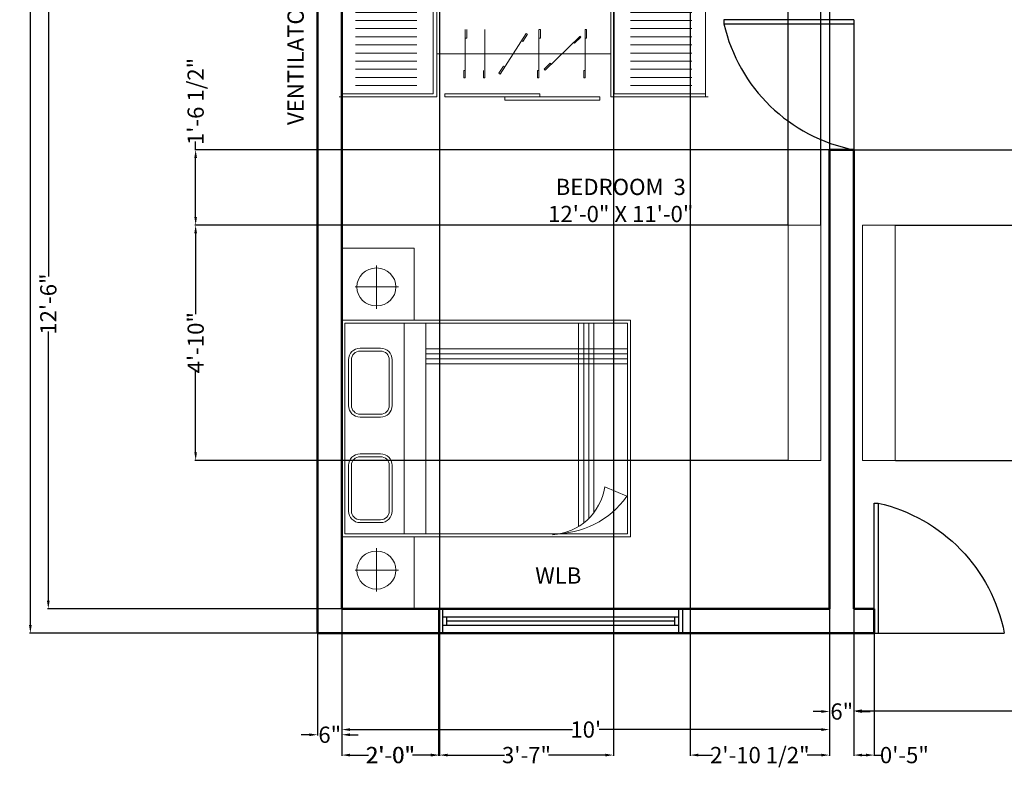
# Model space of a CAD drawing. Units: inches. Extents: x 2663 to 3147, y 140 to 736.
# Tile 1 of 6: x 2663 to 2905, y 140 to 327. Entities that reach past the tile are written whole.
import ezdxf

# ---------------------------------------------------------------- set-up
doc = ezdxf.new("R2010")
doc.units = ezdxf.units.IN
doc.header["$MEASUREMENT"] = 0
for name, color, linetype, lineweight in [('A-ANNO-DIMS', 2, 'Continuous', 18), ('A-AREA-IDEN', 3, 'Continuous', 25), ('A-DOOR', 3, 'Continuous', 25), ('A-FURN', 8, 'Continuous', 18), ('A-GLAZ', 4, 'Continuous', 25), ('A-WALL', 7, 'Continuous', 50)]:
    doc.layers.add(name, color=color, linetype=linetype, lineweight=lineweight)
doc.styles.get("Standard").update_dxf_attribs({"font": 'arial.ttf'})
doc.dimstyles.get("Standard").update_dxf_attribs({"dimtxt": 4, "dimasz": 2, "dimexe": 0.18, "dimexo": 0.0625, "dimgap": 0.09, "dimtad": 0, "dimdec": 0, "dimzin": 0, "dimdsep": 46, "dimlunit": 4, "dimtxsty": 'Standard', "dimcen": 0.09, "dimadec": 0, "dimazin": 0, "dimtfac": 1, "dimtdec": 0, "dimtofl": 0, "dimtmove": 0, "dimatfit": 3, "dimfxl": 1, "dimtolj": 1, "dimtzin": 0, "dimarcsym": 0})

# ---------------------------------------------------------------- blocks, each defined once
blk = doc.blocks.new('*D4')
at = {"layer": 'A-ANNO-DIMS', "color": 0, "lineweight": -2, "transparency": 16777216}
for p, q in [((2742.1, 332.32), (2669.73, 332.32)), ((2669.91, 330.32), (2669.91, 264.1)), ((2669.91, 184.32), (2669.91, 250.55)), ((2742.1, 182.32), (2669.73, 182.32))]:
    blk.add_line(p, q, dxfattribs=at)
at = {"layer": 'A-ANNO-DIMS', "color": 0, "transparency": 16777216}
for points in [[(2669.57, 330.32), (2670.24, 330.32), (2669.91, 332.32)], [(2669.57, 184.32), (2670.24, 184.32), (2669.91, 182.32)]]:
    blk.add_solid(points, dxfattribs=at)
at = {"layer": 'Defpoints', "color": 0, "transparency": 16777216}
for p in [(2669.91, 332.32), (2742.16, 332.32), (2742.16, 182.32)]:
    blk.add_point(p, dxfattribs=at)
at = {"layer": 'A-ANNO-DIMS', "color": 0, "transparency": 16777216, "insert": (2669.91, 257.32), "char_height": 4, "attachment_point": 5, "rotation": 90}
blk.add_mtext('\\A1;12\'-6"', dxfattribs=at)
blk = doc.blocks.new('EDFRTYUI')
for p, q in [((3325.9, 253.54), (3325.9, 259.54)), ((3325.9, 259.54), (3385.9, 259.54)), ((3326.9, 253.54), (3326.9, 259.54)), ((3384.9, 259.54), (3384.9, 253.54)), ((3385.9, 259.54), (3385.9, 253.54)), ((3326.9, 257.54), (3384.9, 257.54)), ((3327.9, 255.54), (3327.9, 257.54)), ((3383.9, 257.54), (3383.9, 255.54)), ((3326.9, 255.54), (3384.9, 255.54)), ((3327.9, 256.54), (3383.9, 256.54)), ((3385.9, 253.54), (3325.9, 253.54))]:
    blk.add_line(p, q)
at = {"insert": (3337.87, 269.72), "char_height": 4, "attachment_point": 1}
blk.add_mtext_dynamic_manual_height_columns('\\pxqc;WLB', width=34.9199, gutter_width=20, heights=[0], dxfattribs=at)
blk = doc.blocks.new('A$C34930FF8')
at = {"ltscale": 0.05}
for p, q in [((0, 2252.4), (0, 16.8)), ((600, 2252.4), (0, 2252.4)), ((185.4, 1513), (185.4, 1521.5)), ((237.7, 1513), (237.7, 1521.5)), ((227.1, 1479.2), (233.2, 1485.2)), ((436.7, 1513), (436.7, 1504.4)), ((482.5, 1513), (482.5, 1504.4)), ((263.6, 1441.7), (269.7, 1447.7)), ((398.2, 1303.6), (392.1, 1297.6)), ((185.4, 1229.1), (185.4, 1237.7)), ((237.7, 1229.1), (237.7, 1237.7)), ((434.8, 1266.1), (428.7, 1260.1)), ((436.7, 1228.2), (436.7, 1219.7)), ((482.5, 1228.2), (482.5, 1219.7)), ((209.5, 1150.1), (214.1, 1157.3)), ((253.5, 1121.8), (258.1, 1129)), ((415.3, 1017.6), (410.6, 1010.5)), ((459.3, 989.3), (454.7, 982.1)), ((482.5, 894.9), (482.5, 886.3)), ((237.7, 775.3), (237.7, 783.9)), ((436.7, 775.3), (436.7, 766.8)), ((482.5, 775.3), (482.5, 766.8)), ((600, 16.8), (0, 16.8))]:
    blk.add_line(p, q, dxfattribs=at)
for p, q in [((580, 1690.9), (580, 2252.4)), ((600, 1669.3), (600, 2269.3)), ((30, 1790.9), (30, 2169.3)), ((80, 1790.9), (80, 2169.3)), ((130, 1790.9), (130, 2169.3)), ((180, 1790.9), (180, 2169.3)), ((230, 1790.9), (230, 2169.3)), ((280, 1790.9), (280, 2169.3)), ((330, 1790.9), (330, 2169.3)), ((380, 1790.9), (380, 2169.3)), ((430, 1790.9), (430, 2169.3)), ((480, 1790.9), (480, 2169.3)), ((530, 1790.9), (530, 2169.3)), ((580, 1690.9), (0, 1690.9)), ((600, 1669.3), (0, 1669.3)), ((335.4, 1666.1), (335.4, 603.1)), ((600, 1603.3), (620, 1603.3)), ((600, 1018.7), (600, 1603.3)), ((620, 1603.3), (620, 1018.7)), ((237.7, 1521.5), (185.4, 1521.5)), ((482.5, 1513), (185.4, 1513)), ((434.8, 1266.1), (227.4, 1478.9)), ((269.7, 1447.7), (233.2, 1485.2)), ((436.7, 1504.4), (482.5, 1504.4)), ((428.7, 1260.1), (392.1, 1297.6)), ((237.7, 1237.7), (185.4, 1237.7)), ((482.5, 1228.2), (185.4, 1228.2)), ((436.7, 1219.7), (482.5, 1219.7)), ((600, 1233.4), (580, 1233.4)), ((580, 1233.4), (580, 648.7)), ((600, 648.7), (600, 1233.4)), ((258.1, 1129), (214.1, 1157.3)), ((459.3, 989.3), (209.5, 1150.1)), ((454.7, 982.1), (410.6, 1010.5)), ((620, 1018.7), (600, 1018.7)), ((482.5, 894.9), (185.4, 894.9)), ((436.7, 886.3), (482.5, 886.3)), ((237.7, 783.9), (185.4, 783.9)), ((482.5, 775.3), (185.4, 775.3)), ((436.7, 766.8), (482.5, 766.8)), ((580, 648.7), (600, 648.7)), ((600, 600), (0, 600)), ((580, 578.3), (0, 578.3)), ((580, 578.3), (580, 16.8)), ((600, 600), (600, 0)), ((30, 478.3), (30, 100)), ((80, 478.3), (80, 100)), ((130, 478.3), (130, 100)), ((180, 478.3), (180, 100)), ((230, 478.3), (230, 100)), ((280, 478.3), (280, 100)), ((330, 478.3), (330, 100)), ((380, 478.3), (380, 100)), ((430, 478.3), (430, 100)), ((480, 478.3), (480, 100)), ((530, 478.3), (530, 100))]:
    blk.add_line(p, q)
blk = doc.blocks.new('A$C057D194F')
for p, q in [((0, 1.5, -0.1688), (0, 2, -0.1688)), ((0, 2, -0.1688), (0.5, 2, -0.1688)), ((0.5, 2, -0.1688), (0.5, 0, -0.1688)), ((2, 2, -0.1688), (0.5, 2, -0.1688)), ((1.98, 1.98, -0.1688), (0.52, 1.98, -0.1688)), ((0.52, 1.98, -0.1688), (0.52, 0.02, -0.1688)), ((1.98, 0.02, -0.1688), (1.98, 1.98, -0.1688)), ((2, 0, -0.1688), (2, 2, -0.1688)), ((2.5, 2, -0.1688), (2, 2, -0.1688)), ((2.5, 1.5, -0.1688), (2.5, 2, -0.1688)), ((1.0907, 1.9539, -0.1688), (0.7735, 1.9539, -0.1688)), ((1.0907, 1.9339, -0.1688), (0.7735, 1.9339, -0.1688)), ((1.8224, 1.9539, -0.1688), (1.5052, 1.9539, -0.1688)), ((1.8224, 1.9339, -0.1688), (1.5052, 1.9339, -0.1688)), ((0.2687, 1.9081, -0.1688), (0.2687, 1.761, -0.1688)), ((0.2687, 1.6081, -0.1688), (0.2687, 1.9081, -0.1688)), ((0.6935, 1.8739, -0.1688), (0.6935, 1.7322, -0.1688)), ((0.7135, 1.8739, -0.1688), (0.7135, 1.7322, -0.1688)), ((1.1507, 1.7322, -0.1688), (1.1507, 1.8739, -0.1688)), ((1.1707, 1.7322, -0.1688), (1.1707, 1.8739, -0.1688)), ((1.4252, 1.8739, -0.1688), (1.4252, 1.7322, -0.1688)), ((1.4452, 1.8739, -0.1688), (1.4452, 1.7322, -0.1688)), ((1.8824, 1.7322, -0.1688), (1.8824, 1.8739, -0.1688)), ((1.9024, 1.7322, -0.1688), (1.9024, 1.8739, -0.1688)), ((2.2313, 1.9081, -0.1688), (2.2313, 1.761, -0.1688)), ((2.2313, 1.6081, -0.1688), (2.2313, 1.9081, -0.1688)), ((0.4194, 1.761, -0.1688), (0.1194, 1.761, -0.1688)), ((0.2687, 1.761, -0.1688), (0.4194, 1.761, -0.1688)), ((0.2687, 1.761, -0.1688), (0.2687, 1.6081, -0.1688)), ((2.0806, 1.761, -0.1688), (2.3806, 1.761, -0.1688)), ((2.2313, 1.761, -0.1688), (2.0806, 1.761, -0.1688)), ((2.2313, 1.761, -0.1688), (2.2313, 1.6081, -0.1688)), ((0.7735, 1.6722, -0.1688), (1.0907, 1.6722, -0.1688)), ((0.7735, 1.6522, -0.1688), (1.0907, 1.6522, -0.1688)), ((1.5052, 1.6722, -0.1688), (1.8224, 1.6722, -0.1688)), ((1.5052, 1.6522, -0.1688), (1.8224, 1.6522, -0.1688)), ((1.98, 1.5693, -0.1688), (0.52, 1.5693, -0.1688)), ((0.5, 1.5, -0.1688), (0, 1.5, -0.1688)), ((2, 1.5, -0.1688), (2.5, 1.5, -0.1688)), ((1.98, 1.4193, -0.1688), (0.52, 1.4193, -0.1688)), ((0.6969, 0.02, -0.1688), (0.6969, 1.4193, -0.1688)), ((0.7319, 0.02, -0.1688), (0.7319, 1.4193, -0.1688)), ((0.7669, 0.02, -0.1688), (0.7669, 1.4193, -0.1688)), ((0.8019, 0.02, -0.1688), (0.8019, 1.4193, -0.1688)), ((0.52, 0.3595, -0.1688), (1.9292, 0.3595, -0.1688)), ((0.52, 0.3245, -0.1688), (1.905, 0.3245, -0.1688)), ((0.52, 0.2895, -0.1688), (1.8742, 0.2895, -0.1688)), ((0.52, 0.2545, -0.1688), (1.8344, 0.2545, -0.1688)), ((1.6548, 0.1789, -0.1688), (1.7198, 0.0251, -0.1688)), ((0.52, 0.02, -0.1688), (1.98, 0.02, -0.1688)), ((0.5, 0, -0.1688), (2, 0, -0.1688))]:
    blk.add_line(p, q)
for centre, radius, start, end in [((0.7735, 1.8739, -0.1688), 0.08, 90, 180), ((0.7735, 1.8739, -0.1688), 0.06, 90, 180), ((1.0907, 1.8739, -0.1688), 0.08, 0, 90), ((1.0907, 1.8739, -0.1688), 0.06, 0, 90), ((1.5052, 1.8739, -0.1688), 0.08, 90, 180), ((1.5052, 1.8739, -0.1688), 0.06, 90, 180), ((1.8224, 1.8739, -0.1688), 0.08, 0, 90), ((1.8224, 1.8739, -0.1688), 0.06, 0, 90), ((0.7735, 1.7322, -0.1688), 0.08, 180, 270), ((0.7735, 1.7322, -0.1688), 0.06, 180, 270), ((1.0907, 1.7322, -0.1688), 0.08, 270, 0), ((1.0907, 1.7322, -0.1688), 0.06, 270, 0), ((1.5052, 1.7322, -0.1688), 0.08, 180, 270), ((1.5052, 1.7322, -0.1688), 0.06, 180, 270), ((1.8224, 1.7322, -0.1688), 0.08, 270, 0), ((1.8224, 1.7322, -0.1688), 0.06, 270, 0), ((1.5992, 0.5623, -0.1688), 0.3874, 278.2518, 356.6808), ((1.363, 0.5286, -0.1688), 0.6171, 305.32946, 1.04595)]:
    blk.add_arc(centre, radius, start, end)
blk.add_ellipse((0.2687, 1.761, -0.1688), major_axis=(0, -0.1351), ratio=0.975448)
at = {"extrusion": (0, 0, -1)}
blk.add_ellipse((2.2313, 1.761, -0.1688), major_axis=(0, 0.1351), ratio=0.975448, dxfattribs=at)
for p in [(0.2687, 1.761, -0.1688), (2.2313, 1.761, -0.1688)]:
    blk.add_point(p)
blk = doc.blocks.new('DXFGVHBJKL')
for p, q in [((2908.16, 532.32), (2907.16, 532.32)), ((2907.16, 532.32), (2907.16, 500.32)), ((2908.16, 500.32), (2908.16, 532.32)), ((2908.16, 500.32), (2876.16, 500.32))]:
    blk.add_line(p, q)
blk.add_arc((2916.21, 492.54), 40.8, 102.812, 169.0067)
blk = doc.blocks.new('*D27')
at = {"layer": 'A-ANNO-DIMS', "color": 0, "lineweight": -2, "transparency": 16777216}
for p, q in [((2868.16, 182.26), (2868.16, 157.05)), ((3090.16, 182.26), (3090.16, 157.05)), ((2870.16, 157.23), (2972.39, 157.23)), ((3088.16, 157.23), (2985.93, 157.23))]:
    blk.add_line(p, q, dxfattribs=at)
at = {"layer": 'A-ANNO-DIMS', "color": 0, "transparency": 16777216}
for points in [[(2870.16, 157.56), (2870.16, 156.89), (2868.16, 157.23)], [(3088.16, 157.56), (3088.16, 156.89), (3090.16, 157.23)]]:
    blk.add_solid(points, dxfattribs=at)
at = {"layer": 'Defpoints', "color": 0, "transparency": 16777216}
for p in [(2868.16, 182.32), (3090.16, 182.32), (2868.16, 157.23)]:
    blk.add_point(p, dxfattribs=at)
at = {"layer": 'A-ANNO-DIMS', "color": 0, "transparency": 16777216, "insert": (2979.16, 157.23), "char_height": 4, "attachment_point": 5}
blk.add_mtext('\\A1;18\'-6"', dxfattribs=at)
blk = doc.blocks.new('*D30')
at = {"layer": 'A-ANNO-DIMS', "color": 0, "lineweight": -2, "transparency": 16777216}
for p, q in [((2862.16, 182.26), (2862.16, 156.87)), ((2868.16, 182.26), (2868.16, 156.87)), ((2860.16, 157.05), (2858.16, 157.05)), ((2870.16, 157.05), (2872.16, 157.05))]:
    blk.add_line(p, q, dxfattribs=at)
at = {"layer": 'A-ANNO-DIMS', "color": 0, "transparency": 16777216}
for points in [[(2860.16, 157.38), (2860.16, 156.71), (2862.16, 157.05)], [(2870.16, 157.38), (2870.16, 156.71), (2868.16, 157.05)]]:
    blk.add_solid(points, dxfattribs=at)
at = {"layer": 'Defpoints', "color": 0, "transparency": 16777216}
for p in [(2862.16, 182.32), (2868.16, 182.32), (2868.16, 157.05)]:
    blk.add_point(p, dxfattribs=at)
at = {"layer": 'A-ANNO-DIMS', "color": 0, "transparency": 16777216, "insert": (2865.16, 157.05), "char_height": 4, "attachment_point": 5}
blk.add_mtext('\\A1;6"', dxfattribs=at)
blk = doc.blocks.new('*D31')
at = {"layer": 'A-ANNO-DIMS', "color": 0, "lineweight": -2, "transparency": 16777216}
for p, q in [((2742.16, 182.26), (2742.16, 152.42)), ((2862.16, 182.26), (2862.16, 152.42)), ((2744.16, 152.6), (2798.87, 152.6)), ((2860.16, 152.6), (2805.46, 152.6))]:
    blk.add_line(p, q, dxfattribs=at)
at = {"layer": 'A-ANNO-DIMS', "color": 0, "transparency": 16777216}
for points in [[(2744.16, 152.93), (2744.16, 152.26), (2742.16, 152.6)], [(2860.16, 152.93), (2860.16, 152.26), (2862.16, 152.6)]]:
    blk.add_solid(points, dxfattribs=at)
at = {"layer": 'Defpoints', "color": 0, "transparency": 16777216}
for p in [(2742.16, 182.32), (2862.16, 182.32), (2742.16, 152.6)]:
    blk.add_point(p, dxfattribs=at)
at = {"layer": 'A-ANNO-DIMS', "color": 0, "transparency": 16777216, "insert": (2802.16, 152.6), "char_height": 4, "attachment_point": 5}
blk.add_mtext("\\A1;10'", dxfattribs=at)
blk = doc.blocks.new('*D32')
at = {"layer": 'A-ANNO-DIMS', "color": 0, "lineweight": -2, "transparency": 16777216}
for p, q in [((2736.16, 182.26), (2736.16, 151.15)), ((2742.16, 182.26), (2742.16, 151.15)), ((2734.16, 151.33), (2732.16, 151.33)), ((2744.16, 151.33), (2746.16, 151.33))]:
    blk.add_line(p, q, dxfattribs=at)
at = {"layer": 'A-ANNO-DIMS', "color": 0, "transparency": 16777216}
for points in [[(2734.16, 151.66), (2734.16, 150.99), (2736.16, 151.33)], [(2744.16, 151.66), (2744.16, 150.99), (2742.16, 151.33)]]:
    blk.add_solid(points, dxfattribs=at)
at = {"layer": 'Defpoints', "color": 0, "transparency": 16777216}
for p in [(2736.16, 182.32), (2742.16, 182.32), (2742.16, 151.33)]:
    blk.add_point(p, dxfattribs=at)
at = {"layer": 'A-ANNO-DIMS', "color": 0, "transparency": 16777216, "insert": (2739.16, 151.33), "char_height": 4, "attachment_point": 5}
blk.add_mtext('\\A1;6"', dxfattribs=at)
blk = doc.blocks.new('*D37')
at = {"layer": 'A-ANNO-DIMS', "color": 0, "lineweight": -2, "transparency": 16777216}
for p, q in [((2736.1, 656.32), (2665.31, 656.32)), ((2665.49, 654.32), (2665.49, 419.89)), ((2665.49, 178.32), (2665.49, 412.76)), ((2736.1, 176.32), (2665.31, 176.32))]:
    blk.add_line(p, q, dxfattribs=at)
at = {"layer": 'A-ANNO-DIMS', "color": 0, "transparency": 16777216}
for points in [[(2665.15, 654.32), (2665.82, 654.32), (2665.49, 656.32)], [(2665.15, 178.32), (2665.82, 178.32), (2665.49, 176.32)]]:
    blk.add_solid(points, dxfattribs=at)
at = {"layer": 'Defpoints', "color": 0, "transparency": 16777216}
for p in [(2665.49, 656.32), (2736.16, 656.32), (2736.16, 176.32)]:
    blk.add_point(p, dxfattribs=at)
at = {"layer": 'A-ANNO-DIMS', "color": 0, "transparency": 16777216, "insert": (2665.49, 416.32), "char_height": 4, "attachment_point": 5, "rotation": 90}
blk.add_mtext("\\A1;40'", dxfattribs=at)
blk = doc.blocks.new('*D43')
at = {"layer": 'A-ANNO-DIMS', "color": 0, "lineweight": -2, "transparency": 16777216}
for p, q in [((2736.1, 399.04), (2730.58, 399.04)), ((2730.76, 397.04), (2730.76, 365.04)), ((2736.1, 363.04), (2730.58, 363.04)), ((2730.76, 363.04), (2730.76, 361.04))]:
    blk.add_line(p, q, dxfattribs=at)
at = {"layer": 'A-ANNO-DIMS', "color": 0, "transparency": 16777216}
for points in [[(2730.43, 397.04), (2731.09, 397.04), (2730.76, 399.04)], [(2730.43, 365.04), (2731.09, 365.04), (2730.76, 363.04)]]:
    blk.add_solid(points, dxfattribs=at)
at = {"layer": 'Defpoints', "color": 0, "transparency": 16777216}
for p in [(2736.16, 399.04), (2730.76, 363.04), (2736.16, 363.04)]:
    blk.add_point(p, dxfattribs=at)
at = {"layer": 'A-ANNO-DIMS', "color": 0, "transparency": 16777216, "insert": (2730.76, 330.34), "char_height": 4, "attachment_point": 5, "rotation": 90}
blk.add_mtext('\\A1;VENTILATOR 3\'-0" TYP.', dxfattribs=at)
blk = doc.blocks.new('*D61')
at = {"layer": 'A-ANNO-DIMS', "color": 0, "lineweight": -2, "transparency": 16777216}
for p, q in [((2851.95, 276.84), (2851.95, 686.5)), ((2853.95, 686.32), (2857.98, 686.32)), ((2859.98, 276.84), (2859.98, 686.5)), ((2859.98, 686.32), (2861.98, 686.32))]:
    blk.add_line(p, q, dxfattribs=at)
at = {"layer": 'A-ANNO-DIMS', "color": 0, "transparency": 16777216}
for points in [[(2853.95, 686.66), (2853.95, 685.99), (2851.95, 686.32)], [(2857.98, 686.66), (2857.98, 685.99), (2859.98, 686.32)]]:
    blk.add_solid(points, dxfattribs=at)
at = {"layer": 'Defpoints', "color": 0, "transparency": 16777216}
for p in [(2859.98, 686.32), (2851.95, 276.78), (2859.98, 276.78)]:
    blk.add_point(p, dxfattribs=at)
at = {"layer": 'A-ANNO-DIMS', "color": 0, "transparency": 16777216, "insert": (2867.39, 686.32), "char_height": 4, "attachment_point": 5}
blk.add_mtext('\\A1;0\'-8"', dxfattribs=at)
blk = doc.blocks.new('*D62')
at = {"layer": 'A-ANNO-DIMS', "color": 0, "lineweight": -2, "transparency": 16777216}
for p, q in [((2851.89, 276.78), (2705.98, 276.78)), ((2706.16, 274.78), (2706.16, 254.86)), ((2706.16, 220.86), (2706.16, 240.78)), ((2851.89, 218.86), (2705.98, 218.86))]:
    blk.add_line(p, q, dxfattribs=at)
at = {"layer": 'A-ANNO-DIMS', "color": 0, "transparency": 16777216}
for points in [[(2705.83, 274.78), (2706.49, 274.78), (2706.16, 276.78)], [(2705.83, 220.86), (2706.49, 220.86), (2706.16, 218.86)]]:
    blk.add_solid(points, dxfattribs=at)
at = {"layer": 'Defpoints', "color": 0, "transparency": 16777216}
for p in [(2706.16, 276.78), (2851.95, 276.78), (2851.95, 218.86)]:
    blk.add_point(p, dxfattribs=at)
at = {"layer": 'A-ANNO-DIMS', "color": 0, "transparency": 16777216, "insert": (2706.16, 247.82), "char_height": 4, "attachment_point": 5, "rotation": 90}
blk.add_mtext('\\A1;4\'-10"', dxfattribs=at)
blk = doc.blocks.new('*D63')
at = {"layer": 'A-ANNO-DIMS', "color": 0, "lineweight": -2, "transparency": 16777216}
for p, q in [((2706.16, 295.32), (2706.16, 297.32)), ((2862.1, 295.32), (2705.98, 295.32)), ((2706.16, 278.78), (2706.16, 293.32)), ((2851.89, 276.78), (2705.98, 276.78))]:
    blk.add_line(p, q, dxfattribs=at)
at = {"layer": 'A-ANNO-DIMS', "color": 0, "transparency": 16777216}
for points in [[(2705.83, 293.32), (2706.49, 293.32), (2706.16, 295.32)], [(2705.83, 278.78), (2706.49, 278.78), (2706.16, 276.78)]]:
    blk.add_solid(points, dxfattribs=at)
at = {"layer": 'Defpoints', "color": 0, "transparency": 16777216}
for p in [(2706.16, 295.32), (2862.16, 295.32), (2851.95, 276.78)]:
    blk.add_point(p, dxfattribs=at)
at = {"layer": 'A-ANNO-DIMS', "color": 0, "transparency": 16777216, "insert": (2706.16, 307.2), "char_height": 4, "attachment_point": 5, "rotation": 90}
blk.add_mtext('\\A1;1\'-6 1/2"', dxfattribs=at)
blk = doc.blocks.new('*D64')
at = {"layer": 'A-ANNO-DIMS', "color": 0, "lineweight": -2, "transparency": 16777216}
for p, q in [((2878.36, 276.78), (3126.34, 276.78)), ((3126.16, 274.78), (3126.16, 254.86)), ((3126.16, 220.86), (3126.16, 240.78)), ((2878.36, 218.86), (3126.34, 218.86))]:
    blk.add_line(p, q, dxfattribs=at)
at = {"layer": 'A-ANNO-DIMS', "color": 0, "transparency": 16777216}
for points in [[(3125.83, 274.78), (3126.49, 274.78), (3126.16, 276.78)], [(3125.83, 220.86), (3126.49, 220.86), (3126.16, 218.86)]]:
    blk.add_solid(points, dxfattribs=at)
at = {"layer": 'Defpoints', "color": 0, "transparency": 16777216}
for p in [(2878.3, 276.78), (3126.16, 276.78), (2878.3, 218.86)]:
    blk.add_point(p, dxfattribs=at)
at = {"layer": 'A-ANNO-DIMS', "color": 0, "transparency": 16777216, "insert": (3126.16, 247.82), "char_height": 4, "attachment_point": 5, "rotation": 90}
blk.add_mtext('\\A1;4\'-10"', dxfattribs=at)
blk = doc.blocks.new('*D65')
at = {"layer": 'A-ANNO-DIMS', "color": 0, "lineweight": -2, "transparency": 16777216}
for p, q in [((3126.16, 295.32), (3126.16, 297.32)), ((2868.22, 295.32), (3126.34, 295.32)), ((3126.16, 278.78), (3126.16, 293.32)), ((2878.36, 276.78), (3126.34, 276.78))]:
    blk.add_line(p, q, dxfattribs=at)
at = {"layer": 'A-ANNO-DIMS', "color": 0, "transparency": 16777216}
for points in [[(3125.83, 293.32), (3126.49, 293.32), (3126.16, 295.32)], [(3125.83, 278.78), (3126.49, 278.78), (3126.16, 276.78)]]:
    blk.add_solid(points, dxfattribs=at)
at = {"layer": 'Defpoints', "color": 0, "transparency": 16777216}
for p in [(2868.16, 295.32), (3126.16, 295.32), (2878.3, 276.78)]:
    blk.add_point(p, dxfattribs=at)
at = {"layer": 'A-ANNO-DIMS', "color": 0, "transparency": 16777216, "insert": (3126.16, 307.2), "char_height": 4, "attachment_point": 5, "rotation": 90}
blk.add_mtext('\\A1;1\'-6 1/2"', dxfattribs=at)
blk = doc.blocks.new('*D70')
at = {"layer": 'A-ANNO-DIMS', "color": 0, "lineweight": -2, "transparency": 16777216}
for p, q in [((2742.16, 182.26), (2742.16, 146.14)), ((2765.96, 182.26), (2765.96, 146.14)), ((2744.16, 146.32), (2748.62, 146.32)), ((2763.96, 146.32), (2759.5, 146.32))]:
    blk.add_line(p, q, dxfattribs=at)
at = {"layer": 'A-ANNO-DIMS', "color": 0, "transparency": 16777216}
for points in [[(2744.16, 146.66), (2744.16, 145.99), (2742.16, 146.32)], [(2763.96, 146.66), (2763.96, 145.99), (2765.96, 146.32)]]:
    blk.add_solid(points, dxfattribs=at)
at = {"layer": 'Defpoints', "color": 0, "transparency": 16777216}
for p in [(2742.16, 182.32), (2765.96, 182.32), (2765.96, 146.32)]:
    blk.add_point(p, dxfattribs=at)
at = {"layer": 'A-ANNO-DIMS', "color": 0, "transparency": 16777216, "insert": (2754.06, 146.32), "char_height": 4, "attachment_point": 5}
blk.add_mtext('\\A1;2\'-0"', dxfattribs=at)
blk = doc.blocks.new('*D71')
at = {"layer": 'A-ANNO-DIMS', "color": 0, "lineweight": -2, "transparency": 16777216}
for p, q in [((2868.16, 182.26), (2868.16, 146.14)), ((2873.16, 182.26), (2873.16, 146.14)), ((2870.16, 146.32), (2871.16, 146.32)), ((2873.16, 146.32), (2875.16, 146.32))]:
    blk.add_line(p, q, dxfattribs=at)
at = {"layer": 'A-ANNO-DIMS', "color": 0, "transparency": 16777216}
for points in [[(2870.16, 146.66), (2870.16, 145.99), (2868.16, 146.32)], [(2871.16, 146.66), (2871.16, 145.99), (2873.16, 146.32)]]:
    blk.add_solid(points, dxfattribs=at)
at = {"layer": 'Defpoints', "color": 0, "transparency": 16777216}
for p in [(2868.16, 182.32), (2873.16, 182.32), (2873.16, 146.32)]:
    blk.add_point(p, dxfattribs=at)
at = {"layer": 'A-ANNO-DIMS', "color": 0, "transparency": 16777216, "insert": (2880.57, 146.32), "char_height": 4, "attachment_point": 5}
blk.add_mtext('\\A1;0\'-5"', dxfattribs=at)
blk = doc.blocks.new('*D81')
at = {"layer": 'A-ANNO-DIMS', "color": 0, "lineweight": -2, "transparency": 16777216}
for p, q in [((2827.83, 410.26), (2827.83, 146.14)), ((2862.16, 410.26), (2862.16, 146.14)), ((2829.83, 146.32), (2833.34, 146.32)), ((2860.16, 146.32), (2856.65, 146.32))]:
    blk.add_line(p, q, dxfattribs=at)
at = {"layer": 'A-ANNO-DIMS', "color": 0, "transparency": 16777216}
for points in [[(2829.83, 146.66), (2829.83, 145.99), (2827.83, 146.32)], [(2860.16, 146.66), (2860.16, 145.99), (2862.16, 146.32)]]:
    blk.add_solid(points, dxfattribs=at)
at = {"layer": 'Defpoints', "color": 0, "transparency": 16777216}
for p in [(2827.83, 410.32), (2862.16, 410.32), (2862.16, 146.32)]:
    blk.add_point(p, dxfattribs=at)
at = {"layer": 'A-ANNO-DIMS', "color": 0, "transparency": 16777216, "insert": (2845, 146.32), "char_height": 4, "attachment_point": 5}
blk.add_mtext('\\A1;2\'-10 1/2"', dxfattribs=at)
blk = doc.blocks.new('*D82')
at = {"layer": 'A-ANNO-DIMS', "color": 0, "lineweight": -2, "transparency": 16777216}
for p, q in [((2742.16, 362.98), (2742.16, 146.14)), ((2766.16, 362.26), (2766.16, 146.14)), ((2744.16, 146.32), (2748.72, 146.32)), ((2764.16, 146.32), (2759.6, 146.32))]:
    blk.add_line(p, q, dxfattribs=at)
at = {"layer": 'A-ANNO-DIMS', "color": 0, "transparency": 16777216}
for points in [[(2744.16, 146.66), (2744.16, 145.99), (2742.16, 146.32)], [(2764.16, 146.66), (2764.16, 145.99), (2766.16, 146.32)]]:
    blk.add_solid(points, dxfattribs=at)
at = {"layer": 'Defpoints', "color": 0, "transparency": 16777216}
for p in [(2742.16, 363.04), (2766.16, 362.32), (2766.16, 146.32)]:
    blk.add_point(p, dxfattribs=at)
at = {"layer": 'A-ANNO-DIMS', "color": 0, "transparency": 16777216, "insert": (2754.16, 146.32), "char_height": 4, "attachment_point": 5}
blk.add_mtext('\\A1;2\'-0"', dxfattribs=at)
blk = doc.blocks.new('*D83')
at = {"layer": 'A-ANNO-DIMS', "color": 0, "lineweight": -2, "transparency": 16777216}
for p, q in [((2766.16, 362.26), (2766.16, 146.14)), ((2808.99, 362.26), (2808.99, 146.14)), ((2768.16, 146.32), (2782.17, 146.32)), ((2806.99, 146.32), (2792.98, 146.32))]:
    blk.add_line(p, q, dxfattribs=at)
at = {"layer": 'A-ANNO-DIMS', "color": 0, "transparency": 16777216}
for points in [[(2768.16, 146.66), (2768.16, 145.99), (2766.16, 146.32)], [(2806.99, 146.66), (2806.99, 145.99), (2808.99, 146.32)]]:
    blk.add_solid(points, dxfattribs=at)
at = {"layer": 'Defpoints', "color": 0, "transparency": 16777216}
for p in [(2766.16, 362.32), (2808.99, 362.32), (2808.99, 146.32)]:
    blk.add_point(p, dxfattribs=at)
at = {"layer": 'A-ANNO-DIMS', "color": 0, "transparency": 16777216, "insert": (2787.58, 146.32), "char_height": 4, "attachment_point": 5}
blk.add_mtext('\\A1;3\'-7"', dxfattribs=at)

msp = doc.modelspace()

# ---------------------------------------------------------------- linework, layer by layer
at = {"layer": 'A-FURN'}
for points in [[(2859.98, 276.78), (2851.95, 276.78), (2851.95, 218.86), (2859.98, 218.86)], [(2870.27, 276.78), (2878.3, 276.78), (2878.3, 218.86), (2870.27, 218.86)]]:
    msp.add_lwpolyline(points, close=True, dxfattribs=at)
at = {"layer": 'A-WALL'}
for p, q in [((2736.16, 176.32), (2736.16, 656.32)), ((2742.16, 182.32), (2742.16, 332.32)), ((2862.16, 182.32), (2862.16, 295.32)), ((2862.16, 295.32), (2868.16, 295.32)), ((2868.16, 182.32), (2868.16, 295.32)), ((2862.16, 182.32), (2742.16, 182.32)), ((2873.16, 182.32), (2868.16, 182.32)), ((2873.16, 176.32), (2873.16, 182.32)), ((2873.16, 176.32), (2736.16, 176.32))]:
    msp.add_line(p, q, dxfattribs=at)

# ---------------------------------------------------------------- block references
at = {"layer": 'A-DOOR', "rotation": 90.00000000000003}
msp.add_blockref('DXFGVHBJKL', (3368.49, -2580.84), dxfattribs=at)
at = {"layer": 'A-DOOR', "xscale": -1}
msp.add_blockref('DXFGVHBJKL', (5781.32, -324), dxfattribs=at)
at = {"layer": 'A-FURN'}
for name, p, xscale, yscale, zscale, rotation in [('A$C34930FF8', (2741.49, 332.32), 0.0400188077054237, 0.0400188077054237, 0.0400188077054237, 270), ('A$C057D194F', (2813.17, 271.08, 5.99), -35.50398587953096, 35.50398587953096, 35.50398587953096, 90)]:
    msp.add_blockref(name, p, dxfattribs=dict(at, xscale=xscale, yscale=yscale, zscale=zscale, rotation=rotation))
at = {"layer": 'A-GLAZ'}
msp.add_blockref('EDFRTYUI', (-559.93, -77.21), dxfattribs=at)

# ---------------------------------------------------------------- texts
at = {"layer": 'A-AREA-IDEN', "insert": (2773.6, 288.17), "char_height": 4, "attachment_point": 1}
msp.add_mtext_dynamic_manual_height_columns('\\pxqc;BEDROOM  3 \\P12\'-0" X 11\'-0"', width=74.3379, gutter_width=20, heights=[0], dxfattribs=at)

# ---------------------------------------------------------------- dimensions: what is measured, and where the dimension line sits
at = {"layer": 'A-ANNO-DIMS'}
for base, p1, p2, override, picture, middle in [((2859.98, 686.32), (2851.95, 276.78), (2859.98, 276.78), {"dimdec": 1, "dimlfac": 1, "dimrnd": 0, "dimzin": 1, "dimdsep": 46, "dimlunit": 4, "dimfrac": 2}, '*D61', (2867.39, 686.32)), ((2862.16, 146.32), (2827.83, 410.32), (2862.16, 410.32), {"dimdec": 1, "dimlfac": 1, "dimrnd": 0, "dimzin": 1, "dimdsep": 46, "dimlunit": 4, "dimfrac": 2}, '*D81', (2845, 146.32)), ((2766.16, 146.32), (2742.16, 363.04), (2766.16, 362.32), {"dimdec": 1, "dimlfac": 1, "dimrnd": 0, "dimzin": 1, "dimdsep": 46, "dimlunit": 4, "dimfrac": 2}, '*D82', (2754.16, 146.32)), ((2808.99, 146.32), (2766.16, 362.32), (2808.99, 362.32), {"dimdec": 1, "dimlfac": 1, "dimrnd": 0, "dimzin": 1, "dimdsep": 46, "dimlunit": 4, "dimfrac": 2}, '*D83', (2787.58, 146.32)), ((2742.16, 151.33), (2736.16, 182.32), (2742.16, 182.32), {"dimclrd": 0, "dimclre": 0, "dimclrt": 0}, '*D32', (2739.16, 151.33)), ((2742.16, 152.6), (2862.16, 182.32), (2742.16, 182.32), {"dimclrd": 0, "dimclre": 0, "dimclrt": 0}, '*D31', (2802.16, 152.6)), ((2765.96, 146.32), (2742.16, 182.32), (2765.96, 182.32), {"dimdec": 1, "dimlfac": 1, "dimrnd": 0, "dimzin": 1, "dimdsep": 46, "dimlunit": 4, "dimfrac": 2}, '*D70', (2754.06, 146.32)), ((2868.16, 157.05), (2862.16, 182.32), (2868.16, 182.32), {"dimclrd": 0, "dimclre": 0, "dimclrt": 0}, '*D30', (2865.16, 157.05)), ((2868.16, 157.23), (3090.16, 182.32), (2868.16, 182.32), {"dimclrd": 0, "dimclre": 0, "dimclrt": 0}, '*D27', (2979.16, 157.23)), ((2873.16, 146.32), (2868.16, 182.32), (2873.16, 182.32), {"dimdec": 1, "dimlfac": 1, "dimrnd": 0, "dimzin": 1, "dimdsep": 46, "dimlunit": 4, "dimfrac": 2}, '*D71', (2880.57, 146.32))]:
    dim = msp.add_linear_dim(base=base, p1=p1, p2=p2, dimstyle='Standard', override=override, dxfattribs=at)
    dim.commit()
    dim.dimension.update_dxf_attribs({"geometry": picture, "text_midpoint": middle})
for base, p1, p2, override, picture, middle in [((2665.49, 656.32), (2736.16, 176.32), (2736.16, 656.32), {"dimclrd": 0, "dimclre": 0, "dimclrt": 0}, '*D37', (2665.49, 416.32)), ((2669.91, 332.32), (2742.16, 182.32), (2742.16, 332.32), {"dimclrd": 0, "dimclre": 0, "dimclrt": 0}, '*D4', (2669.91, 257.32)), ((2706.16, 295.32), (2851.95, 276.78), (2862.16, 295.32), {"dimdec": 1, "dimlfac": 1, "dimrnd": 0, "dimzin": 1, "dimdsep": 46, "dimlunit": 4, "dimfrac": 2}, '*D63', (2706.16, 307.2)), ((3126.16, 295.32), (2878.3, 276.78), (2868.16, 295.32), {"dimdec": 1, "dimlfac": 1, "dimrnd": 0, "dimzin": 1, "dimdsep": 46, "dimlunit": 4, "dimfrac": 2}, '*D65', (3126.16, 307.2)), ((2706.16, 276.78), (2851.95, 218.86), (2851.95, 276.78), {"dimdec": 1, "dimlfac": 1, "dimrnd": 0, "dimzin": 1, "dimdsep": 46, "dimlunit": 4, "dimfrac": 2}, '*D62', (2706.16, 247.82)), ((3126.16, 276.78), (2878.3, 218.86), (2878.3, 276.78), {"dimdec": 1, "dimlfac": 1, "dimrnd": 0, "dimzin": 1, "dimdsep": 46, "dimlunit": 4, "dimfrac": 2}, '*D64', (3126.16, 247.82))]:
    dim = msp.add_linear_dim(base=base, p1=p1, p2=p2, angle=90, dimstyle='Standard', override=override, dxfattribs=at)
    dim.commit()
    dim.dimension.update_dxf_attribs({"geometry": picture, "text_midpoint": middle})
dim = msp.add_linear_dim(base=(2730.76, 363.04), p1=(2736.16, 399.04), p2=(2736.16, 363.04), angle=270, text='VENTILATOR <> TYP.', dimstyle='Standard', override={"dimdec": 1, "dimrnd": 0, "dimzin": 1, "dimlunit": 4, "dimfrac": 2}, dxfattribs=at)
dim.commit()
dim.dimension.update_dxf_attribs({"geometry": '*D43', "text_midpoint": (2730.76, 330.34)})

doc.saveas('drawing.dxf')
